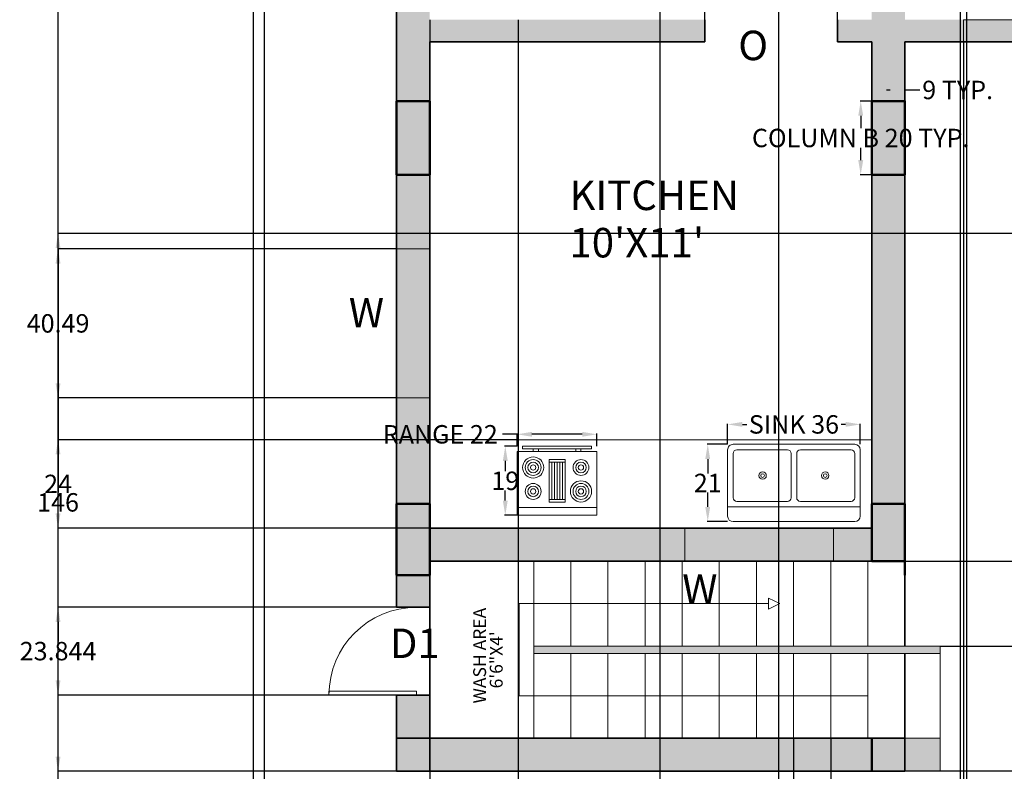
# Model space of a CAD drawing. Units: inches. Extents: x 460 to 1030, y -658 to 271.
# Tile 2 of 10: x 460 to 728, y -486 to -282. Entities that reach past the tile are written whole.
import ezdxf

# ---------------------------------------------------------------- set-up
doc = ezdxf.new("R2010")
doc.units = ezdxf.units.IN
doc.header["$MEASUREMENT"] = 0
doc.linetypes.add('ACAD_ISO02W100', pattern=[15, 12, -3])
for name, color, linetype, lineweight in [('A-ANNO-DIMS', 2, 'Continuous', 18), ('A-ANNO-SYMB', 7, 'Continuous', 18), ('A-ANNO-TEXT', 7, 'Continuous', 18), ('A-AREA-IDEN', 7, 'Continuous', 25), ('A-COLS', 7, 'Continuous', 50), ('A-DOOR', 3, 'Continuous', 20), ('A-EQPM', 8, 'Continuous', 18), ('A-FLOR-CASE', 9, 'Continuous', 18), ('A-FLOR-FIXT', 9, 'Continuous', 18), ('A-FLOR-STRS', 7, 'Continuous', 18), ('A-GLAZ', 4, 'Continuous', 20), ('A-GLAZ-PATT', 4, 'Continuous', 13), ('A-ROOF-OVHD', 8, 'ACAD_ISO02W100', 18), ('A-WALL', 7, 'Continuous', 35), ('A-WALL-PATT', 5, 'Continuous', 13), ('C-PROP', 7, 'Continuous', 25)]:
    doc.layers.add(name, color=color, linetype=linetype, lineweight=lineweight)
doc.layers.add('A-COLS-PATT', color=7, linetype='Continuous', lineweight=13, true_color=0xffffff)
doc.styles.get("Standard").update_dxf_attribs({"font": 'arial.ttf'})
doc.dimstyles.get("Standard").update_dxf_attribs({"dimtxt": 5, "dimasz": 4, "dimexe": 0.18, "dimexo": 0.0625, "dimgap": 0.09, "dimtad": 0, "dimtih": 1, "dimtoh": 1, "dimdec": 1, "dimzin": 0, "dimdsep": 46, "dimlunit": 4, "dimtxsty": 'Standard', "dimcen": 0.09, "dimadec": 0, "dimazin": 0, "dimtfac": 1, "dimtdec": 1, "dimtofl": 0, "dimtmove": 0, "dimatfit": 3, "dimfxl": 1, "dimtolj": 1, "dimtzin": 0, "dimarcsym": 0})

# ---------------------------------------------------------------- blocks, each defined once
blk = doc.blocks.new('Range-Oven - 30 in top')
for p, q in [((0, -3), (30, -3)), ((12, -6), (18, -6)), ((13, -20), (13, -6)), ((14, -6), (14, -20)), ((15, -20), (15, -6)), ((16, -6), (16, -20)), ((17, -20), (17, -6)), ((18, -20), (12, -20)), ((6, -24), (6, -25)), ((8, -25), (8, -24)), ((22, -25), (22, -24)), ((24, -24), (24, -25))]:
    blk.add_line(p, q)
for points in [[(0, -24), (0, 0), (30, 0), (30, -24)], [(12, -21), (12, -5), (18, -5), (18, -21)], [(2, -26), (2, -25), (28, -25), (28, -26)]]:
    blk.add_lwpolyline(points, close=True)
for centre, radius in [((6, -9), 4), ((6, -9), 3), ((6, -9), 2), ((24, -9), 3), ((24, -9), 2), ((6, -9), 1), ((24, -9), 1), ((24, -18), 4), ((6, -18), 3), ((6, -18), 2), ((6, -18), 1), ((24, -18), 3), ((24, -18), 2), ((24, -18), 1)]:
    blk.add_circle(centre, radius)
blk = doc.blocks.new('Sink-double - 36 in top')
for p, q in [((-18, -4), (18, -4)), ((-0.75, -18.5), (-0.75, -6.5)), ((0.75, -6.5), (0.75, -18.5))]:
    blk.add_line(p, q)
for points in [[(-16.5, 0), (16.5, 0)], [(-18, -19.5), (-18, -1.5)], [(18, -1.5), (18, -19.5)], [(-16.5, -18.5), (-16.5, -6.5)], [(-15.5, -5.5), (-1.75, -5.5)], [(1.75, -5.5), (15.5, -5.5)], [(16.5, -6.5), (16.5, -18.5)], [(16.5, -21), (-16.5, -21)], [(-1.75, -19.5), (-15.5, -19.5)], [(15.5, -19.5), (1.75, -19.5)]]:
    blk.add_lwpolyline(points)
for centre, radius in [((-8.5, -12.5), 1), ((-8.5, -12.5), 0.5), ((8.5, -12.5), 1), ((8.5, -12.5), 0.5)]:
    blk.add_circle(centre, radius)
for centre, radius, start, end in [((-16.5, -1.5), 1.5, 90, 180), ((16.5, -1.5), 1.5, 0, 90), ((-15.5, -6.5), 1, 90, 180), ((-1.75, -6.5), 1, 0, 90), ((1.75, -6.5), 1, 90, 180), ((15.5, -6.5), 1, 0, 90), ((-15.5, -18.5), 1, 180, 270), ((-1.75, -18.5), 1, 270, 0), ((1.75, -18.5), 1, 180, 270), ((15.5, -18.5), 1, 270, 0), ((-16.5, -19.5), 1.5, 180, 270), ((16.5, -19.5), 1.5, 270, 0)]:
    blk.add_arc(centre, radius, start, end)
blk = doc.blocks.new('*U2')
for p, q in [((0, 0), (0, -6)), ((40, 0), (40, -6))]:
    blk.add_line(p, q)
blk.add_lwpolyline([(0, 0), (0, 40), (1.75, 40), (1.75, 0)], close=True)
blk.add_arc((0, 0), 40, 0, 90)
blk = doc.blocks.new('COL-RECT-TYPE-B')
blk.add_lwpolyline([(0, 0), (-9, 0), (-9, 20.04), (0, 20.04)], close=True)
blk = doc.blocks.new('*D21')
at = {"layer": 'A-ANNO-DIMS', "color": 0, "lineweight": -2, "transparency": 16777216}
for p, q in [((691.73, -303.81), (688.61, -303.81)), ((688.79, -307.81), (688.79, -311.15)), ((688.79, -319.84), (688.79, -316.5)), ((691.73, -323.84), (688.61, -323.84))]:
    blk.add_line(p, q, dxfattribs=at)
at = {"layer": 'A-ANNO-DIMS', "color": 0, "transparency": 16777216}
for points in [[(688.12, -307.81), (689.46, -307.81), (688.79, -303.81)], [(688.12, -319.84), (689.46, -319.84), (688.79, -323.84)]]:
    blk.add_solid(points, dxfattribs=at)
at = {"layer": 'Defpoints', "color": 0, "transparency": 16777216}
for p in [(688.79, -303.81), (691.8, -303.81), (691.8, -323.84)]:
    blk.add_point(p, dxfattribs=at)
at = {"layer": 'A-ANNO-DIMS', "color": 0, "transparency": 16777216, "insert": (688.79, -313.83), "char_height": 5, "attachment_point": 5}
blk.add_mtext('\\A1;COLUMN B 20 TYP.', dxfattribs=at)
blk = doc.blocks.new('*D22')
at = {"layer": 'A-ANNO-DIMS', "color": 0, "lineweight": -2, "transparency": 16777216}
for p, q in [((691.8, -303.75), (691.8, -300.62)), ((695.8, -300.8), (696.8, -300.8)), ((700.8, -303.75), (700.8, -300.62)), ((700.8, -300.8), (704.8, -300.8))]:
    blk.add_line(p, q, dxfattribs=at)
at = {"layer": 'A-ANNO-DIMS', "color": 0, "transparency": 16777216}
for points in [[(695.8, -300.14), (695.8, -301.47), (691.8, -300.8)], [(696.8, -300.14), (696.8, -301.47), (700.8, -300.8)]]:
    blk.add_solid(points, dxfattribs=at)
at = {"layer": 'Defpoints', "color": 0, "transparency": 16777216}
for p in [(700.8, -300.8), (691.8, -303.81), (700.8, -303.81)]:
    blk.add_point(p, dxfattribs=at)
at = {"layer": 'A-ANNO-DIMS', "color": 0, "transparency": 16777216, "insert": (715.11, -300.8), "char_height": 5, "attachment_point": 5}
blk.add_mtext('\\A1;9 TYP.', dxfattribs=at)
blk = doc.blocks.new('*D31')
at = {"layer": 'A-ANNO-DIMS', "color": 0, "lineweight": -2, "transparency": 16777216}
for p, q in [((595.53, -394.26), (591.53, -394.26)), ((595.53, -397.44), (595.53, -394.08)), ((613.17, -394.26), (599.53, -394.26)), ((617.17, -397.44), (617.17, -394.08))]:
    blk.add_line(p, q, dxfattribs=at)
at = {"layer": 'A-ANNO-DIMS', "color": 0, "transparency": 16777216}
for points in [[(599.53, -393.59), (599.53, -394.92), (595.53, -394.26)], [(613.17, -393.59), (613.17, -394.92), (617.17, -394.26)]]:
    blk.add_solid(points, dxfattribs=at)
at = {"layer": 'Defpoints', "color": 0, "transparency": 16777216}
for p in [(595.53, -394.26), (595.53, -397.5), (617.17, -397.5)]:
    blk.add_point(p, dxfattribs=at)
at = {"layer": 'A-ANNO-DIMS', "color": 0, "transparency": 16777216, "insert": (574.63, -394.26), "char_height": 5, "attachment_point": 5}
blk.add_mtext('\\A1;RANGE 22', dxfattribs=at)
blk = doc.blocks.new('*D32')
at = {"layer": 'A-ANNO-DIMS', "color": 0, "lineweight": -2, "transparency": 16777216}
for p, q in [((595.47, -397.5), (592.11, -397.5)), ((592.29, -401.5), (592.29, -404.23)), ((592.29, -412.25), (592.29, -409.52)), ((595.47, -416.25), (592.11, -416.25))]:
    blk.add_line(p, q, dxfattribs=at)
at = {"layer": 'A-ANNO-DIMS', "color": 0, "transparency": 16777216}
for points in [[(591.62, -401.5), (592.96, -401.5), (592.29, -397.5)], [(591.62, -412.25), (592.96, -412.25), (592.29, -416.25)]]:
    blk.add_solid(points, dxfattribs=at)
at = {"layer": 'Defpoints', "color": 0, "transparency": 16777216}
for p in [(595.53, -397.5), (592.29, -416.25), (595.53, -416.25)]:
    blk.add_point(p, dxfattribs=at)
at = {"layer": 'A-ANNO-DIMS', "color": 0, "transparency": 16777216, "insert": (592.29, -406.88), "char_height": 5, "attachment_point": 5}
blk.add_mtext('\\A1;19', dxfattribs=at)
blk = doc.blocks.new('*D33')
at = {"layer": 'A-ANNO-DIMS', "color": 0, "lineweight": -2, "transparency": 16777216}
for p, q in [((652.66, -396.9), (652.66, -391.39)), ((656.66, -391.57), (657.88, -391.57)), ((684.66, -391.57), (683.44, -391.57)), ((688.66, -396.9), (688.66, -391.39))]:
    blk.add_line(p, q, dxfattribs=at)
at = {"layer": 'A-ANNO-DIMS', "color": 0, "transparency": 16777216}
for points in [[(656.66, -390.9), (656.66, -392.23), (652.66, -391.57)], [(684.66, -390.9), (684.66, -392.23), (688.66, -391.57)]]:
    blk.add_solid(points, dxfattribs=at)
at = {"layer": 'Defpoints', "color": 0, "transparency": 16777216}
for p in [(652.66, -391.57), (652.66, -396.97), (688.66, -396.97)]:
    blk.add_point(p, dxfattribs=at)
at = {"layer": 'A-ANNO-DIMS', "color": 0, "transparency": 16777216, "insert": (670.66, -391.57), "char_height": 5, "attachment_point": 5}
blk.add_mtext('\\A1;SINK 36', dxfattribs=at)
blk = doc.blocks.new('*D34')
at = {"layer": 'A-ANNO-DIMS', "color": 0, "lineweight": -2, "transparency": 16777216}
for p, q in [((652.59, -396.97), (647.08, -396.97)), ((647.26, -400.97), (647.26, -404.87)), ((647.26, -413.97), (647.26, -410.07)), ((652.59, -417.97), (647.08, -417.97))]:
    blk.add_line(p, q, dxfattribs=at)
at = {"layer": 'A-ANNO-DIMS', "color": 0, "transparency": 16777216}
for points in [[(646.59, -400.97), (647.92, -400.97), (647.26, -396.97)], [(646.59, -413.97), (647.92, -413.97), (647.26, -417.97)]]:
    blk.add_solid(points, dxfattribs=at)
at = {"layer": 'Defpoints', "color": 0, "transparency": 16777216}
for p in [(652.66, -396.97), (647.26, -417.97), (652.66, -417.97)]:
    blk.add_point(p, dxfattribs=at)
at = {"layer": 'A-ANNO-DIMS', "color": 0, "transparency": 16777216, "insert": (647.26, -407.47), "char_height": 5, "attachment_point": 5}
blk.add_mtext('\\A1;21', dxfattribs=at)
blk = doc.blocks.new('*D40')
at = {"layer": 'A-ANNO-DIMS', "color": 0, "lineweight": -2, "transparency": 16777216}
for p, q in [((523.73, 201.27), (470.68, 201.27)), ((470.86, 197.27), (470.86, -202.58)), ((470.86, -607.73), (470.86, -207.87)), ((523.73, -611.73), (470.68, -611.73))]:
    blk.add_line(p, q, dxfattribs=at)
at = {"layer": 'A-ANNO-DIMS', "color": 0, "transparency": 16777216}
for points in [[(470.19, 197.27), (471.52, 197.27), (470.86, 201.27)], [(470.19, -607.73), (471.52, -607.73), (470.86, -611.73)]]:
    blk.add_solid(points, dxfattribs=at)
at = {"layer": 'Defpoints', "color": 0, "transparency": 16777216}
for p in [(470.86, 201.27), (523.8, 201.27), (523.8, -611.73)]:
    blk.add_point(p, dxfattribs=at)
at = {"layer": 'A-ANNO-DIMS', "color": 0, "transparency": 16777216, "insert": (470.86, -205.23), "char_height": 5, "attachment_point": 5}
blk.add_mtext('\\A1;813', dxfattribs=at)
blk = doc.blocks.new('*D50')
at = {"layer": 'A-ANNO-DIMS', "color": 0, "lineweight": -2, "transparency": 16777216}
for p, q in [((700.86, -428.73), (1022.03, -428.73)), ((1021.85, -432.73), (1021.85, -437.58)), ((1021.85, -447.73), (1021.85, -442.87)), ((710.38, -451.73), (1022.03, -451.73))]:
    blk.add_line(p, q, dxfattribs=at)
at = {"layer": 'A-ANNO-DIMS', "color": 0, "transparency": 16777216}
for points in [[(1021.18, -432.73), (1022.51, -432.73), (1021.85, -428.73)], [(1021.18, -447.73), (1022.51, -447.73), (1021.85, -451.73)]]:
    blk.add_solid(points, dxfattribs=at)
at = {"layer": 'Defpoints', "color": 0, "transparency": 16777216}
for p in [(700.8, -428.73), (710.32, -451.73), (1021.85, -451.73)]:
    blk.add_point(p, dxfattribs=at)
at = {"layer": 'A-ANNO-DIMS', "color": 0, "transparency": 16777216, "insert": (1021.85, -440.23), "char_height": 5, "attachment_point": 5}
blk.add_mtext('\\A1;23', dxfattribs=at)
blk = doc.blocks.new('*D51')
at = {"layer": 'A-ANNO-DIMS', "color": 0, "lineweight": -2, "transparency": 16777216}
for p, q in [((670.56, -476.79), (670.56, -654.61)), ((680.64, -476.79), (680.64, -654.61)), ((674.56, -654.43), (676.64, -654.43)), ((680.64, -654.43), (684.64, -654.43))]:
    blk.add_line(p, q, dxfattribs=at)
at = {"layer": 'A-ANNO-DIMS', "color": 0, "transparency": 16777216}
for points in [[(674.56, -653.77), (674.56, -655.1), (670.56, -654.43)], [(676.64, -653.77), (676.64, -655.1), (680.64, -654.43)]]:
    blk.add_solid(points, dxfattribs=at)
at = {"layer": 'Defpoints', "color": 0, "transparency": 16777216}
for p in [(670.56, -476.73), (680.64, -476.73), (680.64, -654.43)]:
    blk.add_point(p, dxfattribs=at)
at = {"layer": 'A-ANNO-DIMS', "color": 0, "transparency": 16777216, "insert": (694.88, -654.43), "char_height": 5, "attachment_point": 5}
blk.add_mtext('\\A1;10.079', dxfattribs=at)
blk = doc.blocks.new('*D57')
at = {"layer": 'A-ANNO-DIMS', "color": 0, "lineweight": -2, "transparency": 16777216}
for p, q in [((717.53, -38.79), (717.53, -654.61)), ((741.59, -38.79), (741.59, -654.61)), ((713.53, -654.43), (709.53, -654.43)), ((745.59, -654.43), (749.59, -654.43))]:
    blk.add_line(p, q, dxfattribs=at)
at = {"layer": 'A-ANNO-DIMS', "color": 0, "transparency": 16777216}
for points in [[(713.53, -653.77), (713.53, -655.1), (717.53, -654.43)], [(745.59, -653.77), (745.59, -655.1), (741.59, -654.43)]]:
    blk.add_solid(points, dxfattribs=at)
at = {"layer": 'Defpoints', "color": 0, "transparency": 16777216}
for p in [(717.53, -38.73), (741.59, -38.73), (741.59, -654.43)]:
    blk.add_point(p, dxfattribs=at)
at = {"layer": 'A-ANNO-DIMS', "color": 0, "transparency": 16777216, "insert": (729.56, -654.43), "char_height": 5, "attachment_point": 5}
blk.add_mtext('\\A1;24.065', dxfattribs=at)
blk = doc.blocks.new('*D61')
at = {"layer": 'A-ANNO-DIMS', "color": 0, "lineweight": -2, "transparency": 16777216}
for p, q in [((646.47, -287.66), (646.47, 267.89)), ((650.47, 267.71), (660.81, 267.71)), ((678.47, 267.71), (668.14, 267.71)), ((682.47, -287.66), (682.47, 267.89))]:
    blk.add_line(p, q, dxfattribs=at)
at = {"layer": 'A-ANNO-DIMS', "color": 0, "transparency": 16777216}
for points in [[(650.47, 268.38), (650.47, 267.04), (646.47, 267.71)], [(678.47, 268.38), (678.47, 267.04), (682.47, 267.71)]]:
    blk.add_solid(points, dxfattribs=at)
at = {"layer": 'Defpoints', "color": 0, "transparency": 16777216}
for p in [(682.47, 267.71), (646.47, -287.73), (682.47, -287.73)]:
    blk.add_point(p, dxfattribs=at)
at = {"layer": 'A-ANNO-DIMS', "color": 0, "transparency": 16777216, "insert": (664.47, 267.71), "char_height": 5, "attachment_point": 5}
blk.add_mtext('\\A1;36', dxfattribs=at)
blk = doc.blocks.new('*D63')
at = {"layer": 'A-ANNO-DIMS', "color": 0, "lineweight": -2, "transparency": 16777216}
for p, q in [((571.8, -281.79), (571.8, -654.61)), ((595.8, -281.79), (595.8, -654.61)), ((575.8, -654.43), (580.09, -654.43)), ((591.8, -654.43), (587.5, -654.43))]:
    blk.add_line(p, q, dxfattribs=at)
at = {"layer": 'A-ANNO-DIMS', "color": 0, "transparency": 16777216}
for points in [[(575.8, -653.77), (575.8, -655.1), (571.8, -654.43)], [(591.8, -653.77), (591.8, -655.1), (595.8, -654.43)]]:
    blk.add_solid(points, dxfattribs=at)
at = {"layer": 'Defpoints', "color": 0, "transparency": 16777216}
for p in [(571.8, -281.73), (595.8, -281.73), (595.8, -654.43)]:
    blk.add_point(p, dxfattribs=at)
at = {"layer": 'A-ANNO-DIMS', "color": 0, "transparency": 16777216, "insert": (583.8, -654.43), "char_height": 5, "attachment_point": 5}
blk.add_mtext('\\A1;24', dxfattribs=at)
blk = doc.blocks.new('*D65')
at = {"layer": 'A-ANNO-DIMS', "color": 0, "lineweight": -2, "transparency": 16777216}
for p, q in [((595.73, -395.73), (470.68, -395.73)), ((470.86, -399.73), (470.86, -405.13)), ((470.86, -415.73), (470.86, -410.33)), ((571.73, -419.73), (470.68, -419.73))]:
    blk.add_line(p, q, dxfattribs=at)
at = {"layer": 'A-ANNO-DIMS', "color": 0, "transparency": 16777216}
for points in [[(470.19, -399.73), (471.52, -399.73), (470.86, -395.73)], [(470.19, -415.73), (471.52, -415.73), (470.86, -419.73)]]:
    blk.add_solid(points, dxfattribs=at)
at = {"layer": 'Defpoints', "color": 0, "transparency": 16777216}
for p in [(470.86, -395.73), (595.8, -395.73), (571.8, -419.73)]:
    blk.add_point(p, dxfattribs=at)
at = {"layer": 'A-ANNO-DIMS', "color": 0, "transparency": 16777216, "insert": (470.86, -407.73), "char_height": 5, "attachment_point": 5}
blk.add_mtext('\\A1;24', dxfattribs=at)
blk = doc.blocks.new('*D66')
at = {"layer": 'A-ANNO-DIMS', "color": 0, "lineweight": -2, "transparency": 16777216}
for p, q in [((940.73, -339.73), (470.68, -339.73)), ((470.86, -343.73), (470.86, -410.08)), ((470.86, -481.73), (470.86, -415.37)), ((979.73, -485.73), (470.68, -485.73))]:
    blk.add_line(p, q, dxfattribs=at)
at = {"layer": 'A-ANNO-DIMS', "color": 0, "transparency": 16777216}
for points in [[(470.19, -343.73), (471.52, -343.73), (470.86, -339.73)], [(470.19, -481.73), (471.52, -481.73), (470.86, -485.73)]]:
    blk.add_solid(points, dxfattribs=at)
at = {"layer": 'Defpoints', "color": 0, "transparency": 16777216}
for p in [(940.8, -339.73), (470.86, -485.73), (979.8, -485.73)]:
    blk.add_point(p, dxfattribs=at)
at = {"layer": 'A-ANNO-DIMS', "color": 0, "transparency": 16777216, "insert": (470.86, -412.73), "char_height": 5, "attachment_point": 5}
blk.add_mtext('\\A1;146', dxfattribs=at)
blk = doc.blocks.new('*D68')
at = {"layer": 'A-ANNO-DIMS', "color": 0, "lineweight": -2, "transparency": 16777216}
for p, q in [((634.27, 90.21), (634.27, -654.61)), ((666.46, 90.21), (666.46, -654.61)), ((638.27, -654.43), (639.91, -654.43)), ((662.46, -654.43), (660.82, -654.43))]:
    blk.add_line(p, q, dxfattribs=at)
at = {"layer": 'A-ANNO-DIMS', "color": 0, "transparency": 16777216}
for points in [[(638.27, -653.77), (638.27, -655.1), (634.27, -654.43)], [(662.46, -653.77), (662.46, -655.1), (666.46, -654.43)]]:
    blk.add_solid(points, dxfattribs=at)
at = {"layer": 'Defpoints', "color": 0, "transparency": 16777216}
for p in [(634.27, 90.27), (666.46, 90.27), (666.46, -654.43)]:
    blk.add_point(p, dxfattribs=at)
at = {"layer": 'A-ANNO-DIMS', "color": 0, "transparency": 16777216, "insert": (650.37, -654.43), "char_height": 5, "attachment_point": 5}
blk.add_mtext('\\A1;32.184', dxfattribs=at)
blk = doc.blocks.new('*D70')
at = {"layer": 'A-ANNO-DIMS', "color": 0, "lineweight": -2, "transparency": 16777216}
for p, q in [((716.71, -287.79), (716.71, -654.61)), ((789.82, -287.79), (789.82, -654.61)), ((720.71, -654.43), (744.79, -654.43)), ((785.82, -654.43), (761.75, -654.43))]:
    blk.add_line(p, q, dxfattribs=at)
at = {"layer": 'A-ANNO-DIMS', "color": 0, "transparency": 16777216}
for points in [[(720.71, -653.77), (720.71, -655.1), (716.71, -654.43)], [(785.82, -653.77), (785.82, -655.1), (789.82, -654.43)]]:
    blk.add_solid(points, dxfattribs=at)
at = {"layer": 'Defpoints', "color": 0, "transparency": 16777216}
for p in [(716.71, -287.73), (789.82, -287.73), (789.82, -654.43)]:
    blk.add_point(p, dxfattribs=at)
at = {"layer": 'A-ANNO-DIMS', "color": 0, "transparency": 16777216, "insert": (753.27, -654.43), "char_height": 5, "attachment_point": 5}
blk.add_mtext('\\A1;73.12', dxfattribs=at)
blk = doc.blocks.new('*D72')
at = {"layer": 'A-ANNO-DIMS', "color": 0, "lineweight": -2, "transparency": 16777216}
for p, q in [((715.8, 68.25), (715.8, -654.61)), ((748.8, 57.75), (748.8, -654.61)), ((719.8, -654.43), (728.63, -654.43)), ((744.8, -654.43), (735.97, -654.43))]:
    blk.add_line(p, q, dxfattribs=at)
at = {"layer": 'A-ANNO-DIMS', "color": 0, "transparency": 16777216}
for points in [[(719.8, -653.77), (719.8, -655.1), (715.8, -654.43)], [(744.8, -653.77), (744.8, -655.1), (748.8, -654.43)]]:
    blk.add_solid(points, dxfattribs=at)
at = {"layer": 'Defpoints', "color": 0, "transparency": 16777216}
for p in [(715.8, 68.31), (748.8, 57.81), (748.8, -654.43)]:
    blk.add_point(p, dxfattribs=at)
at = {"layer": 'A-ANNO-DIMS', "color": 0, "transparency": 16777216, "insert": (732.3, -654.43), "char_height": 5, "attachment_point": 5}
blk.add_mtext('\\A1;33', dxfattribs=at)
blk = doc.blocks.new('*D76')
at = {"layer": 'A-ANNO-DIMS', "color": 0, "lineweight": -2, "transparency": 16777216}
for p, q in [((562.73, -343.9), (470.68, -343.9)), ((470.86, -347.9), (470.86, -361.51)), ((470.86, -380.4), (470.86, -366.79)), ((562.73, -384.4), (470.68, -384.4))]:
    blk.add_line(p, q, dxfattribs=at)
at = {"layer": 'A-ANNO-DIMS', "color": 0, "transparency": 16777216}
for points in [[(470.19, -347.9), (471.52, -347.9), (470.86, -343.9)], [(470.19, -380.4), (471.52, -380.4), (470.86, -384.4)]]:
    blk.add_solid(points, dxfattribs=at)
at = {"layer": 'Defpoints', "color": 0, "transparency": 16777216}
for p in [(562.8, -343.9), (470.86, -384.4), (562.8, -384.4)]:
    blk.add_point(p, dxfattribs=at)
at = {"layer": 'A-ANNO-DIMS', "color": 0, "transparency": 16777216, "insert": (470.86, -364.15), "char_height": 5, "attachment_point": 5}
blk.add_mtext('\\A1;40.49', dxfattribs=at)
blk = doc.blocks.new('*D77')
at = {"layer": 'A-ANNO-DIMS', "color": 0, "lineweight": -2, "transparency": 16777216}
for p, q in [((562.73, -441.19), (470.68, -441.19)), ((470.86, -445.19), (470.86, -450.47)), ((470.86, -461.03), (470.86, -455.76)), ((562.73, -465.03), (470.68, -465.03))]:
    blk.add_line(p, q, dxfattribs=at)
at = {"layer": 'A-ANNO-DIMS', "color": 0, "transparency": 16777216}
for points in [[(470.19, -445.19), (471.52, -445.19), (470.86, -441.19)], [(470.19, -461.03), (471.52, -461.03), (470.86, -465.03)]]:
    blk.add_solid(points, dxfattribs=at)
at = {"layer": 'Defpoints', "color": 0, "transparency": 16777216}
for p in [(562.8, -441.19), (470.86, -465.03), (562.8, -465.03)]:
    blk.add_point(p, dxfattribs=at)
at = {"layer": 'A-ANNO-DIMS', "color": 0, "transparency": 16777216, "insert": (470.86, -453.11), "char_height": 5, "attachment_point": 5}
blk.add_mtext('\\A1;23.844', dxfattribs=at)

msp = doc.modelspace()

# ---------------------------------------------------------------- hatches: boundary and pattern name
at = {"layer": 'A-COLS-PATT'}
h = msp.add_hatch(color=256, dxfattribs=at)
h.dxf.hatch_style = 1
h.paths.add_polyline_path([(571.7961, 90.2738), (562.7961, 90.2738), (562.7961, 71.6966), (571.7961, 71.6966)])
h.paths.add_polyline_path([(700.7961, 90.2738), (691.7961, 90.2738), (691.7961, 71.6966), (700.7961, 71.6966)])
h.paths.add_polyline_path([(811.7961, 90.2738), (802.7961, 90.2738), (802.7961, 71.6966), (811.7961, 71.6966)])
h.paths.add_polyline_path([(940.7961, 90.2738), (931.7961, 90.2738), (931.7961, 71.6966), (940.7961, 71.6966)])
h.paths.add_polyline_path([(940.7961, -101.149), (931.7961, -101.149), (931.7961, -119.7262), (940.7961, -119.7262)])
h.paths.add_polyline_path([(940.7961, -268.3723), (931.7961, -268.3723), (931.7961, -287.7262), (940.7961, -287.7262)])
h.paths.add_polyline_path([(803.0275, -281.7262), (789.8237, -281.7262), (789.8237, -287.7262), (803.0275, -287.7262)])
h.paths.add_polyline_path([(700.7961, -303.809), (691.7961, -303.809), (691.7961, -323.8443), (700.7961, -323.8443)])
h.paths.add_polyline_path([(571.7961, -303.809), (562.7961, -303.809), (562.7961, -323.8443), (571.7961, -323.8443)])
h.paths.add_polyline_path([(571.7961, -413.1453), (562.7961, -413.1453), (562.7961, -432.4659), (571.7961, -432.4659)])
h.paths.add_polyline_path([(571.7961, -101.149), (562.7961, -101.149), (562.7961, -119.7262), (571.7961, -119.7262)])
h.paths.add_polyline_path([(700.7961, -101.0985), (691.7961, -101.0985), (691.7961, -119.7262), (700.7961, -119.7262)])
h.paths.add_polyline_path([(811.7961, -101.149), (802.7961, -101.149), (802.7961, -119.7262), (811.7961, -119.7262)])
h = msp.add_hatch(color=256, dxfattribs=at)
h.dxf.hatch_style = 1
h.paths.add_polyline_path([(700.7961, -413.1453), (691.7961, -413.1453), (691.7961, -428.7262), (700.7961, -428.7262)])
h = msp.add_hatch(color=256, dxfattribs=at)
h.dxf.hatch_style = 1
h.paths.add_polyline_path([(700.7961, -476.7262), (691.7961, -476.7262), (691.7961, -485.7262), (700.7961, -485.7262)])
h.paths.add_polyline_path([(571.7961, -476.7262), (562.7961, -476.7262), (562.7961, -485.7262), (571.7961, -485.7262)])
at = {"layer": 'A-GLAZ-PATT'}
h = msp.add_hatch(color=256, dxfattribs=at)
h.dxf.hatch_style = 1
h.paths.add_polyline_path([(571.7961, -343.9041), (562.7961, -343.9041), (562.7961, -384.3969), (571.7961, -384.3969)])
h.paths.add_polyline_path([(571.7961, -143.2895), (562.7961, -143.2895), (562.7961, -168.3798), (571.7961, -168.3798)])
h.paths.add_polyline_path([(571.7961, -49.2966), (562.7961, -49.2966), (562.7961, -90.3192), (571.7961, -90.3192)])
h.paths.add_polyline_path([(666.4584, 90.2738), (634.2742, 90.2738), (634.2742, 81.2738), (666.4584, 81.2738)])
h.paths.add_polyline_path([(742.1779, 90.2738), (713.201, 90.2738), (713.201, 81.2738), (742.1779, 81.2738)])
h.paths.add_polyline_path([(797.2395, 90.2738), (768.2626, 90.2738), (768.2626, 81.2738), (797.2395, 81.2738)])
h.paths.add_polyline_path([(918.7723, 90.2738), (881.2728, 90.2738), (881.2728, 81.2738), (918.7723, 81.2738)])
h.paths.add_polyline_path([(940.7961, -60.0042), (931.7961, -60.0042), (931.7961, -95.7262), (940.7961, -95.7262)])
h.paths.add_polyline_path([(940.7961, -163.6558), (931.7961, -163.6558), (931.7961, -230.2946), (940.7961, -230.2946)])
h.paths.add_polyline_path([(913.7961, -331.7262), (835.7961, -331.7262), (835.7961, -332.7262), (913.7961, -332.7262)])
h.paths.add_polyline_path([(871.4559, -281.7262), (831.4302, -281.7262), (831.4302, -287.7262), (871.4559, -287.7262)])
h.paths.add_polyline_path([(774.8576, -281.7262), (716.7073, -281.7262), (716.7073, -287.7262), (774.8576, -287.7262)])
h = msp.add_hatch(color=256, dxfattribs=at)
h.dxf.hatch_style = 1
h.paths.add_polyline_path([(681.4044, -419.7262), (641.0603, -419.7262), (641.0603, -428.7262), (681.4044, -428.7262)])
at = {"layer": 'A-WALL-PATT'}
h = msp.add_hatch(color=256, dxfattribs=at)
h.dxf.hatch_style = 1
h.paths.add_polyline_path([(634.2742, 90.2738), (571.7961, 90.2738), (571.7961, 81.2738), (634.2742, 81.2738)])
h.paths.add_polyline_path([(691.7961, 90.2738), (666.4584, 90.2738), (666.4584, 81.2738), (691.7961, 81.2738)])
h.paths.add_polyline_path([(713.201, 90.2738), (700.7961, 90.2738), (700.7961, 81.2738), (713.201, 81.2738)])
h.paths.add_polyline_path([(748.7961, 90.2738), (742.1779, 90.2738), (742.1779, 81.2738), (748.7961, 81.2738)])
h.paths.add_polyline_path([(768.2626, 90.2738), (754.7961, 90.2738), (754.7961, 81.2738), (768.2626, 81.2738)])
h.paths.add_polyline_path([(802.7961, 90.2738), (797.2395, 90.2738), (797.2395, 81.2738), (802.7961, 81.2738)])
h.paths.add_polyline_path([(881.2728, 90.2738), (811.7961, 90.2738), (811.7961, 81.2738), (881.2728, 81.2738)])
h.paths.add_polyline_path([(931.7961, 90.2738), (918.7723, 90.2738), (918.7723, 81.2738), (931.7961, 81.2738)])
h.paths.add_polyline_path([(940.7961, 71.6966), (931.7961, 71.6966), (931.7961, -60.0042), (940.7961, -60.0042)])
h.paths.add_polyline_path([(940.7961, -95.7262), (931.7961, -95.7262), (931.7961, -101.149), (940.7961, -101.149)])
h.paths.add_polyline_path([(931.7961, -110.7262), (894.6225, -110.7262), (894.6225, -119.7262), (931.7961, -119.7262)])
h.paths.add_polyline_path([(858.6225, -110.7262), (811.7961, -110.7262), (811.7961, -119.7262), (858.6225, -119.7262)])
h.paths.add_polyline_path([(940.7961, -119.7262), (931.7961, -119.7262), (931.7961, -141.7212), (931.7961, -163.6558), (940.7961, -163.6558)])
h.paths.add_polyline_path([(940.7961, -230.2946), (931.7961, -230.2946), (931.7961, -268.3723), (940.7961, -268.3723)])
h.paths.add_polyline_path([(931.7961, -281.7262), (908.3452, -281.7262), (908.3452, -285.0181), (908.3452, -287.7262), (931.7961, -287.7262)])
h.paths.add_polyline_path([(831.4302, -281.7262), (803.0275, -281.7262), (803.0275, -287.7262), (808.7961, -287.7262), (808.7961, -339.7262), (811.7961, -339.7262), (811.7961, -287.7262), (831.4302, -287.7262)])
h.paths.add_polyline_path([(789.8237, -281.7262), (774.8576, -281.7262), (774.8576, -287.7262), (789.8237, -287.7262)])
h.paths.add_polyline_path([(716.7073, -281.7262), (700.7961, -281.7262), (700.7961, -271.1977), (691.7961, -271.1977), (691.7961, -281.7262), (682.4735, -281.7262), (682.4735, -287.7262), (691.7961, -287.7262), (691.7961, -303.809), (700.7961, -303.809), (700.7961, -287.7262), (716.7073, -287.7262)])
h.paths.add_polyline_path([(700.7961, -323.8443), (691.7961, -323.8443), (691.7961, -413.1453), (700.7961, -413.1453)])
h.paths.add_polyline_path([(940.7961, -287.7262), (937.7961, -287.7262), (937.7961, -339.7262), (940.7961, -339.7262)])
h.paths.add_polyline_path([(937.7961, -336.7262), (811.7961, -336.7262), (811.7961, -339.7262), (937.7961, -339.7262)])
h.paths.add_polyline_path([(835.7961, -329.7262), (811.7961, -329.7262), (811.7961, -332.7262), (835.7961, -332.7262)])
h.paths.add_polyline_path([(937.7961, -329.7262), (913.7961, -329.7262), (913.7961, -332.7262), (937.7961, -332.7262)])
h.paths.add_polyline_path([(691.7961, -419.7262), (681.4044, -419.7262), (681.4044, -428.7262), (691.7961, -428.7262)])
h.paths.add_polyline_path([(691.7961, -476.7262), (571.7961, -476.7262), (571.7961, -485.7262), (691.7961, -485.7262)])
h.paths.add_polyline_path([(571.7961, -465.0348), (568.223, -465.0348), (562.7961, -465.0348), (562.7961, -476.7262), (571.7961, -476.7262)])
h.paths.add_polyline_path([(571.7961, -432.4659), (562.7961, -432.4659), (562.7961, -441.1912), (571.7961, -441.1912)])
h.paths.add_polyline_path([(571.7961, -384.3969), (562.7961, -384.3969), (562.7961, -413.1453), (571.7961, -413.1453)])
h.paths.add_polyline_path([(571.7961, -323.8443), (562.7961, -323.8443), (562.7961, -343.9041), (571.7961, -343.9041)])
h.paths.add_polyline_path([(571.7961, -287.7262), (646.4735, -287.7262), (646.4735, -281.7262), (571.7961, -281.7262), (571.7961, -258.1542), (571.7961, -233.7262), (566.4164, -233.7262), (562.7961, -233.7262), (562.7961, -303.809), (571.7961, -303.809)])
h.paths.add_polyline_path([(571.7961, -179.7262), (691.7961, -179.7262), (691.7961, -197.5753), (700.7961, -197.5753), (700.7961, -173.7262), (647.7961, -173.7262), (647.7961, -165.5723), (643.7961, -165.5723), (643.7961, -173.7262), (571.7961, -173.7262), (571.7961, -168.3798), (562.7961, -168.3798), (562.7961, -197.7262), (571.7961, -197.7262)])
h.paths.add_polyline_path([(647.7961, -110.7262), (571.7961, -110.7262), (571.7961, -119.7262), (643.7961, -119.7262), (643.7961, -141.5723), (647.7961, -141.5723)])
h.paths.add_polyline_path([(691.7961, -110.7262), (683.7961, -110.7262), (683.7961, -114.3453), (683.7961, -119.7262), (691.7961, -119.7262)])
h.paths.add_polyline_path([(571.7961, -119.7262), (562.7961, -119.7262), (562.7961, -143.2895), (571.7961, -143.2895)])
h.paths.add_polyline_path([(571.7961, -90.3192), (562.7961, -90.3192), (562.7961, -101.149), (571.7961, -101.149)])
h.paths.add_polyline_path([(571.7961, 71.6966), (562.7961, 71.6966), (562.7961, -49.2966), (571.7961, -49.2966)])
h.paths.add_polyline_path([(700.7961, 71.6966), (691.7961, 71.6966), (691.7961, -50.298), (700.7961, -50.298)])
h.paths.add_polyline_path([(754.7961, 81.2738), (748.7961, 81.2738), (748.7961, -38.7262), (741.5908, -38.7262), (741.5908, -39.109), (741.5908, -42.7262), (748.7961, -42.7262), (748.7961, -110.7262), (754.7961, -110.7262), (754.7961, -42.7262), (773.6274, -42.7262), (773.6274, -38.7262), (754.7961, -38.7262)])
h.paths.add_polyline_path([(717.4759, -38.7262), (700.7961, -38.7262), (700.7961, -42.7262), (717.4759, -42.7262)])
h.paths.add_polyline_path([(811.7961, 71.6966), (802.7961, 71.6966), (802.7961, -50.298), (811.7961, -50.298)])
h.paths.add_polyline_path([(811.7961, -86.298), (806.4164, -86.298), (802.7961, -86.298), (802.7961, -101.149), (811.7961, -101.149)])
h = msp.add_hatch(color=256, dxfattribs=at)
h.dxf.hatch_style = 1
h.paths.add_polyline_path([(641.0603, -419.7262), (571.7961, -419.7262), (571.7961, -428.7262), (641.0603, -428.7262)])
h = msp.add_hatch(color=256, dxfattribs=at)
h.dxf.hatch_style = 1
h.paths.add_polyline_path([(710.3211, -451.7262), (600.0072, -451.7262), (600.0072, -453.7262), (710.3211, -453.7262)])
h.paths.add_polyline_path([(710.3211, -476.7262), (700.7961, -476.7262), (700.7961, -485.7262), (710.3211, -485.7262)])

# ---------------------------------------------------------------- linework, layer by layer
at = {"layer": 'A-ANNO-SYMB'}
for p, q in [((610.0861, -440.2262), (596.0172, -440.2262)), ((596.0172, -440.2262), (596.0172, -465.2262)), ((610.0861, -440.2262), (663.7814, -440.2262)), ((596.0172, -465.2262), (690.7172, -465.2262))]:
    msp.add_line(p, q, dxfattribs=at)
msp.add_lwpolyline([(663.7814, -441.707), (666.8074, -440.2262), (663.7814, -438.7454), (663.7814, -440.2262)], close=True, dxfattribs=at)
at = {"layer": 'A-COLS'}
for p, q in [((691.7961, -428.7262), (700.7961, -428.7262)), ((691.7961, -476.7262), (691.7961, -485.7262))]:
    msp.add_line(p, q, dxfattribs=at)
msp.add_lwpolyline([(571.7961, -432.4659), (562.7961, -432.4659), (562.7961, -413.1453), (571.7961, -413.1453)], close=True, dxfattribs=at)
msp.add_lwpolyline([(691.7961, -428.7262), (691.7961, -413.1453), (700.7961, -413.1453), (700.7961, -432.4659)], dxfattribs=at)
at = {"layer": 'A-FLOR-CASE'}
for p, q in [((595.7961, -287.7262), (595.7961, -395.7262)), ((595.7961, -395.7262), (691.7961, -395.7262))]:
    msp.add_line(p, q, dxfattribs=at)
at = {"layer": 'A-FLOR-STRS'}
for p, q in [((600.0072, -428.7262), (600.0072, -476.7262)), ((610.0861, -428.7262), (610.0861, -451.7262)), ((620.165, -428.7262), (620.165, -451.7262)), ((630.2439, -428.7262), (630.2439, -451.7262)), ((640.3227, -428.7262), (640.3227, -451.7262)), ((650.4016, -428.7262), (650.4016, -451.7262)), ((660.4805, -428.7262), (660.4805, -451.7262)), ((670.5594, -428.7262), (670.5594, -451.7262)), ((680.6383, -428.7262), (680.6383, -451.7262)), ((690.7172, -428.7262), (690.7172, -451.7262)), ((600.0072, -451.7262), (710.3211, -451.7262)), ((710.3211, -451.7262), (710.3211, -476.7262)), ((600.0072, -453.7262), (710.3211, -453.7262)), ((610.0861, -453.7262), (610.0861, -476.7262)), ((620.165, -453.7262), (620.165, -476.7262)), ((630.2439, -453.7262), (630.2439, -476.7262)), ((640.3227, -453.7262), (640.3227, -476.7262)), ((650.4016, -453.7262), (650.4016, -476.7262)), ((660.4805, -453.7262), (660.4805, -476.7262)), ((670.5594, -453.7262), (670.5594, -476.7262)), ((680.6383, -453.7262), (680.6383, -476.7262)), ((690.7172, -453.7262), (690.7172, -476.7262)), ((710.3211, -476.7262), (700.7961, -476.7262)), ((710.3211, -476.7262), (710.3211, -485.7262)), ((710.3211, -485.7262), (709.7505, -485.7262))]:
    msp.add_line(p, q, dxfattribs=at)
at = {"layer": 'A-GLAZ'}
for points in [[(716.7073, -281.7262), (774.8576, -281.7262), (774.8576, -287.7262), (716.7073, -287.7262)], [(571.7961, -343.9041), (562.7961, -343.9041), (562.7961, -384.3969), (571.7961, -384.3969)], [(681.4044, -428.7262), (641.0603, -428.7262), (641.0603, -419.7262), (681.4044, -419.7262)]]:
    msp.add_lwpolyline(points, close=True, dxfattribs=at)
at = {"layer": 'A-ROOF-OVHD'}
msp.add_line((976.7961, -485.7262), (700.7961, -485.7262), dxfattribs=at)
at = {"layer": 'A-WALL'}
for p, q in [((562.7961, -233.7262), (562.7961, -441.1912)), ((646.4735, -287.7262), (646.4735, -281.7262)), ((682.4735, -281.7262), (682.4735, -287.7262)), ((571.7961, -287.7262), (571.7961, -485.7262)), ((646.4735, -287.7262), (571.7961, -287.7262)), ((691.7961, -287.7262), (682.4735, -287.7262)), ((691.7961, -287.7262), (691.7961, -428.7262)), ((691.7961, -287.7262), (691.7961, -413.1453)), ((808.7961, -287.7262), (700.7961, -287.7262)), ((700.7961, -287.7262), (700.7961, -451.7262)), ((691.7961, -419.7262), (571.7961, -419.7262)), ((691.7961, -428.7262), (571.7961, -428.7262)), ((571.7961, -441.1912), (562.7961, -441.1912)), ((700.7961, -453.7262), (700.7961, -485.7262)), ((562.7961, -465.0348), (571.7961, -465.0348)), ((562.7961, -465.0348), (562.7961, -485.7262)), ((700.7961, -476.7262), (562.7961, -476.7262)), ((691.7961, -485.7262), (562.7961, -485.7262)), ((700.7961, -485.7262), (691.7961, -485.7262))]:
    msp.add_line(p, q, dxfattribs=at)
at = {"layer": 'C-PROP'}
for p, q in [((523.7961, 129.2738), (523.7961, -524.7262)), ((526.7961, 126.2738), (526.7961, -608.7262))]:
    msp.add_line(p, q, dxfattribs=at)

# ---------------------------------------------------------------- block references
at = {"layer": 'A-COLS'}
for p in [(571.7961, -323.8443), (700.7961, -323.8443)]:
    msp.add_blockref('COL-RECT-TYPE-B', p, dxfattribs=at)
at = {"layer": 'A-DOOR', "xscale": 0.5955130742725966, "yscale": 0.5955130742725966, "zscale": 0.5955130742725966, "rotation": 90.00000000000003}
msp.add_blockref('*U2', (568.223, -465.0348), dxfattribs=at)
at = {"layer": 'A-EQPM', "xscale": 0.72111010717278, "yscale": 0.72111010717278, "zscale": 0.72111010717278, "rotation": 180}
msp.add_blockref('Range-Oven - 30 in top', (617.1681, -416.2511), dxfattribs=at)
at = {"layer": 'A-FLOR-FIXT', "rotation": 180}
msp.add_blockref('Sink-double - 36 in top', (670.657, -417.9662), dxfattribs=at)

# ---------------------------------------------------------------- texts
at = {"layer": 'A-ANNO-TEXT'}
for s, p in [('O', (655.547, -292.7116)), ('W', (549.7936, -365.2314)), ('W', (640.3227, -440.2262)), ('D1', (560.9249, -454.9882))]:
    msp.add_text(s, height=8, dxfattribs=at).set_placement(p)
at = {"layer": 'A-AREA-IDEN'}
for s, p in [('KITCHEN', (609.7096, -333.3998)), ("10'X11'", (609.7096, -346.2511))]:
    msp.add_text(s, height=8, dxfattribs=at).set_placement(p)
for s, p in [('WASH AREA', (587.0655, -467.3162)), ('6\'6"X4\'', (591.573, -463.2271))]:
    msp.add_text(s, height=3.47917, rotation=90, dxfattribs=at).set_placement(p)

# ---------------------------------------------------------------- dimensions: what is measured, and where the dimension line sits
at = {"layer": 'A-ANNO-DIMS'}
for base, p1, p2, override, picture, middle in [((682.4735, 267.7108), (646.4735, -287.7262), (682.4735, -287.7262), {"dimdec": 0, "dimlfac": 1, "dimrnd": 0, "dimzin": 0, "dimdsep": 46, "dimlunit": 2}, '*D61', (664.4735, 267.7108)), ((666.4584, -654.4339), (634.2742, 90.2738), (666.4584, 90.2738), {"dimdec": 3, "dimlfac": 1, "dimrnd": 0, "dimzin": 0, "dimdsep": 46, "dimlunit": 2}, '*D68', (650.3663, -654.4339)), ((748.7961, -654.4339), (715.7961, 68.3148), (748.7961, 57.8148), {"dimdec": 0, "dimlfac": 1, "dimrnd": 0, "dimzin": 0, "dimdsep": 46, "dimlunit": 2}, '*D72', (732.2961, -654.4339)), ((741.5908, -654.4339), (717.5258, -38.7262), (741.5908, -38.7262), {"dimdec": 3, "dimlfac": 1, "dimrnd": 0, "dimzin": 0, "dimdsep": 46, "dimlunit": 2}, '*D57', (729.5583, -654.4339)), ((595.7961, -654.4339), (571.7961, -281.7262), (595.7961, -281.7262), {"dimdec": 0, "dimlfac": 1, "dimrnd": 0, "dimzin": 0, "dimdsep": 46, "dimlunit": 2}, '*D63', (583.7961, -654.4339)), ((789.8237, -654.4339), (716.7073, -287.7262), (789.8237, -287.7262), {"dimdec": 2, "dimlfac": 1, "dimrnd": 0, "dimzin": 0, "dimdsep": 46, "dimlunit": 2}, '*D70', (753.2655, -654.4339)), ((680.6383, -654.4339), (670.5594, -476.7262), (680.6383, -476.7262), {"dimdec": 3, "dimlfac": 1, "dimrnd": 0, "dimzin": 0, "dimdsep": 46, "dimlunit": 2}, '*D51', (694.8767, -654.4339))]:
    dim = msp.add_linear_dim(base=base, p1=p1, p2=p2, dimstyle='Standard', override=override, dxfattribs=at)
    dim.commit()
    dim.dimension.update_dxf_attribs({"geometry": picture, "text_midpoint": middle})
for base, p1, p2, angle, override, picture, middle in [((470.8563, 201.2738), (523.7961, -611.7262), (523.7961, 201.2738), 90, {"dimdec": 0, "dimlfac": 1, "dimrnd": 0, "dimzin": 0, "dimdsep": 46, "dimlunit": 2}, '*D40', (470.8563, -205.2262)), ((470.8563, -485.7262), (940.7961, -339.7262), (979.7961, -485.7262), 90, {"dimdec": 0, "dimlfac": 1, "dimrnd": 0, "dimzin": 0, "dimdsep": 46, "dimlunit": 2}, '*D66', (470.8563, -412.7262)), ((470.8563, -384.3969), (562.7961, -343.9041), (562.7961, -384.3969), 90, {"dimdec": 2, "dimlfac": 1, "dimrnd": 0, "dimzin": 0, "dimdsep": 46, "dimlunit": 2}, '*D76', (470.8563, -364.1505)), ((470.8563, -395.7262), (571.7961, -419.7262), (595.7961, -395.7262), 90, {"dimdec": 0, "dimlfac": 1, "dimrnd": 0, "dimzin": 0, "dimdsep": 46, "dimlunit": 2}, '*D65', (470.8563, -407.7262)), ((592.2898, -416.2511), (595.5348, -397.5023), (595.5348, -416.2511), 270, {"dimdec": 0, "dimlfac": 1, "dimrnd": 0, "dimzin": 0, "dimdsep": 46, "dimlunit": 2}, '*D32', (592.2898, -406.8767)), ((647.257, -417.9662), (652.657, -396.9662), (652.657, -417.9662), 270, {"dimdec": 0, "dimlfac": 1, "dimrnd": 0, "dimzin": 0, "dimdsep": 46, "dimlunit": 2}, '*D34', (647.257, -407.4662)), ((1021.8461, -451.7262), (700.7961, -428.7262), (710.3211, -451.7262), 90, {"dimdec": 0, "dimlfac": 1, "dimrnd": 0, "dimzin": 0, "dimdsep": 46, "dimlunit": 2}, '*D50', (1021.8461, -440.2262)), ((470.8563, -465.0348), (562.7961, -441.1912), (562.7961, -465.0348), 90, {"dimdec": 3, "dimlfac": 1, "dimrnd": 0, "dimzin": 0, "dimdsep": 46, "dimlunit": 2}, '*D77', (470.8563, -453.113))]:
    dim = msp.add_linear_dim(base=base, p1=p1, p2=p2, angle=angle, dimstyle='Standard', override=override, dxfattribs=at)
    dim.commit()
    dim.dimension.update_dxf_attribs({"geometry": picture, "text_midpoint": middle})
dim = msp.add_linear_dim(base=(700.7961, -300.8038), p1=(691.7961, -303.809), p2=(700.7961, -303.809), text='<> TYP.', dimstyle='Standard', override={"dimdec": 0, "dimlfac": 1, "dimrnd": 0, "dimzin": 0, "dimdsep": 46, "dimlunit": 2}, dxfattribs=at)
dim.commit()
dim.dimension.update_dxf_attribs({"geometry": '*D22', "text_midpoint": (715.1129, -300.8038)})
for base, p1, p2, angle, text, picture, middle in [((688.7908, -303.809), (691.7961, -323.8443), (691.7961, -303.809), 90, 'COLUMN B <> TYP.', '*D21', (688.7908, -313.8266)), ((652.657, -391.5662), (688.657, -396.9662), (652.657, -396.9662), 180, 'SINK <>', '*D33', (670.657, -391.5662)), ((595.5348, -394.2573), (617.1681, -397.5023), (595.5348, -397.5023), 180, 'RANGE <>', '*D31', (574.6287, -394.2573))]:
    dim = msp.add_linear_dim(base=base, p1=p1, p2=p2, angle=angle, text=text, dimstyle='Standard', override={"dimdec": 0, "dimlfac": 1, "dimrnd": 0, "dimzin": 0, "dimdsep": 46, "dimlunit": 2}, dxfattribs=at)
    dim.commit()
    dim.dimension.update_dxf_attribs({"geometry": picture, "text_midpoint": middle})

doc.saveas('drawing.dxf')
